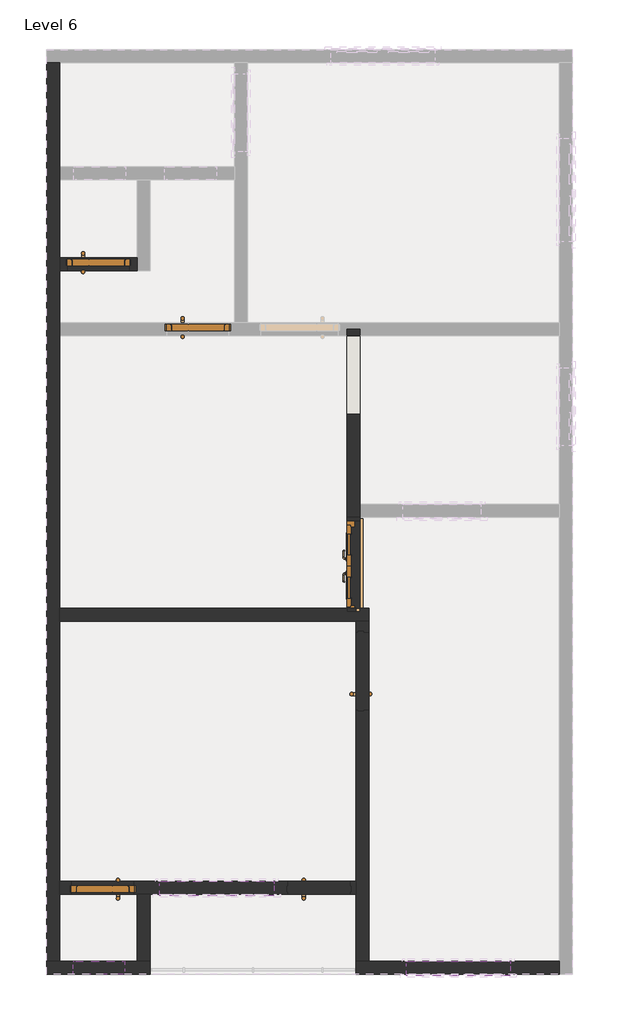
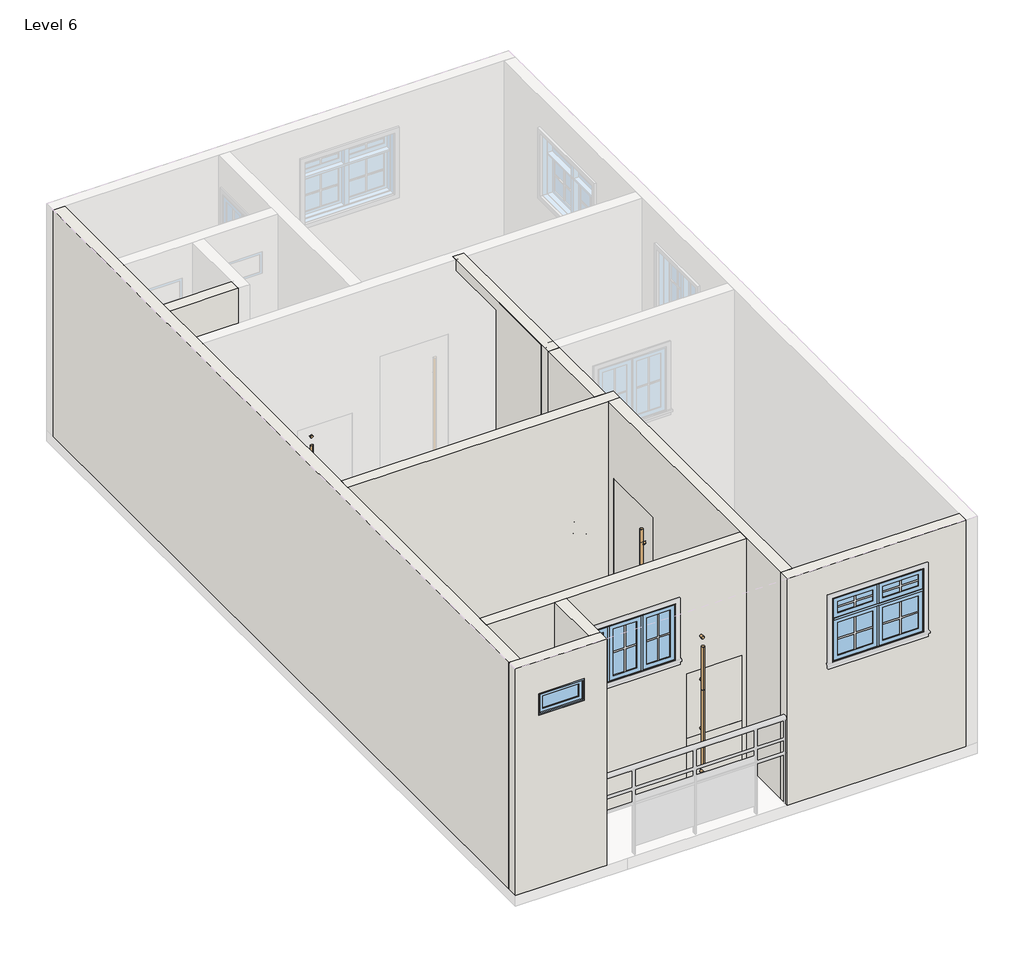
# One storey, part 1 of 3: 31 walls, 7 doors, 6 windows.
"""IFC4 building model written with IfcOpenShell, lengths in millimetres."""

from ifc_helpers import new_model, si_unit, frame, origin, place, context, project, spatial, polyline, outline, extrude, faceted_brep, transform, mapped, element, save
from components import door_9b787682, door_dc81b0c5, door_3_5c4206ef, door_2576ec39, door_55c03dfd, fixed_2_65c13adb, window_61697a4f, m_window_casement_double_awning_double_4_7efa9bbd

model = new_model("IFC4")

# Units and contexts
model_context = context("Model", 3, world=origin())
ifc_project = project(units=[si_unit("LENGTHUNIT", "METRE", prefix="MILLI")], contexts=[model_context])

# Site, building, storey
site = spatial("IfcSite", under=ifc_project)
building = spatial("IfcBuilding", under=site)
storey = spatial("IfcBuildingStorey", under=building, Name="Level 6", Elevation=7010.4)

# Doors
placement = place(None, origin())
door_shape = door_9b787682(model_context)
element("IfcDoor", 1, ObjectType="2'5\"", at=placement, inside=storey, context=model_context, shape_type="MappedRepresentation", body=[
    mapped(door_shape, transform((-22033.2963079, 3049.4742053, 7010.4), x_axis=(1.0, 0.0, 0.0), y_axis=(0.0, 1.0, 0.0), z_axis=(0.0, 0.0, 1.0))),
])
element("IfcDoor", 2, ObjectType="2'5\"", at=placement, inside=storey, context=model_context, shape_type="MappedRepresentation", body=[
    mapped(door_shape, transform((-23201.6963079, 3811.4742053, 7010.4), x_axis=(1.0, 0.0, 0.0), y_axis=(0.0, 1.0, 0.0), z_axis=(0.0, 0.0, 1.0))),
])
element("IfcDoor", 3, ObjectType="2'5\"", at=placement, inside=storey, context=model_context, shape_type="MappedRepresentation", body=[
    mapped(door_shape, transform((-23150.8963079, -3503.7257947, 7010.4), x_axis=(-1.0, 0.0, 0.0), y_axis=(0.0, -1.0, 0.0), z_axis=(0.0, 0.0, 1.0))),
])
door_2_shape = door_dc81b0c5(model_context)
element("IfcDoor", 4, ObjectType="2'5\"", at=placement, inside=storey, context=model_context, shape_type="MappedRepresentation", body=[
    mapped(door_2_shape, transform((-20610.8963079, -3503.7257947, 7056.6445349), x_axis=(1.0, 0.0, 0.0), y_axis=(0.0, 1.0, 0.0), z_axis=(0.0, 0.0, 1.0))),
])
element("IfcDoor", 5, ObjectType="2'5\"", at=placement, inside=storey, context=model_context, shape_type="MappedRepresentation", body=[
    mapped(door_2_shape, transform((-20610.8963079, -3503.7257947, 7666.2445349), x_axis=(1.0, 0.0, 0.0), y_axis=(0.0, 1.0, 0.0), z_axis=(0.0, 0.0, 1.0))),
])
door_3_shape = door_3_5c4206ef(model_context)
element("IfcDoor", 6, ObjectType="3'", at=placement, inside=storey, context=model_context, shape_type="MappedRepresentation", body=[
    mapped(door_3_shape, transform((-20102.8963079, -963.7257947, 7010.4), x_axis=(0.0, 1.0, 0.0), y_axis=(-1.0, 0.0, 0.0), z_axis=(0.0, 0.0, 1.0))),
])
door_4_shape = door_2576ec39(model_context)
door_5_shape = door_55c03dfd(model_context)
element("IfcDoor", 7, ObjectType="ExtDbl (8) : 3'6\"", at=placement, inside=storey, context=model_context, shape_type="MappedRepresentation", body=[
    mapped(door_4_shape, transform((-20204.4963079, 268.1742053, 7010.4), x_axis=(0.0, -1.0, 0.0), y_axis=(1.0, 0.0, 0.0), z_axis=(0.0, 0.0, 1.0))),
    mapped(door_5_shape, transform((-20204.4963079, 268.1742053, 7010.4), x_axis=(0.0, -1.0, 0.0), y_axis=(1.0, 0.0, 0.0), z_axis=(0.0, 0.0, 1.0))),
])

# Walls
element("IfcWall", 8, ObjectType="Generic - 6\"", at=placement, inside=storey, context=model_context, shape_type="Brep", body=[
    faceted_brep([(-17791.4963079, -4367.3257947, 7010.4), (-20026.6963079, -4367.3257947, 7010.4), (-20179.0963079, -4367.3257947, 7010.4), (-20179.0963079, -4367.3257947, 10210.8), (-20026.6963079, -4367.3257947, 10210.8), (-17791.4963079, -4367.3257947, 10210.8), (-19585.5697454, -4367.3257947, 9739.2), (-19585.5697454, -4367.3257947, 8839.2), (-18366.3697454, -4367.3257947, 8839.2), (-18366.3697454, -4367.3257947, 9739.2), (-17791.4963079, -4519.7257947, 7010.4), (-17791.4963079, -4519.7257947, 10210.8), (-20179.0963079, -4519.7257947, 10210.8), (-20179.0963079, -4519.7257947, 7010.4), (-19585.5697454, -4519.7257947, 9739.2), (-18366.3697454, -4519.7257947, 9739.2), (-18366.3697454, -4519.7257947, 8839.2), (-19585.5697454, -4519.7257947, 8839.2)], [[[0, 1, 2, 3, 4, 5], [6, 7, 8, 9]], [[10, 11, 12, 13], [14, 15, 16, 17]], [[2, 1, 0, 10, 13]], [[5, 4, 3, 12, 11]], [[0, 5, 11, 10]], [[3, 2, 13, 12]], [[7, 6, 14, 17]], [[8, 7, 17, 16]], [[9, 8, 16, 15]], [[6, 9, 15, 14]]]),
])
element("IfcWall", 9, ObjectType="Generic - 6\"", at=placement, inside=storey, context=model_context, shape_type="Brep", body=[
    faceted_brep([(-23811.2963079, -4519.7257947, 7010.4), (-22592.0963079, -4519.7257947, 7010.4), (-22592.0963079, -4519.7257947, 10210.8), (-23811.2963079, -4519.7257947, 10210.8), (-23500.5431829, -4519.7257947, 9753.6), (-22890.9431829, -4519.7257947, 9753.6), (-22890.9431829, -4519.7257947, 9448.8), (-23500.5431829, -4519.7257947, 9448.8), (-23811.2963079, -4367.3257947, 7010.4), (-23811.2963079, -4367.3257947, 10210.8), (-23658.8963079, -4367.3257947, 10210.8), (-22744.4963079, -4367.3257947, 10210.8), (-22592.0963079, -4367.3257947, 10210.8), (-22592.0963079, -4367.3257947, 7010.4), (-22744.4963079, -4367.3257947, 7010.4), (-23658.8963079, -4367.3257947, 7010.4), (-23500.5431829, -4367.3257947, 9753.6), (-23500.5431829, -4367.3257947, 9448.8), (-22890.9431829, -4367.3257947, 9448.8), (-22890.9431829, -4367.3257947, 9753.6)], [[[0, 1, 2, 3], [4, 5, 6, 7]], [[8, 9, 10, 11, 12, 13, 14, 15], [16, 17, 18, 19]], [[1, 0, 8, 15, 14, 13]], [[3, 2, 12, 11, 10, 9]], [[0, 3, 9, 8]], [[2, 1, 13, 12]], [[17, 16, 4, 7]], [[18, 17, 7, 6]], [[19, 18, 6, 5]], [[16, 19, 5, 4]]]),
])
element("IfcWall", 10, ObjectType="Generic - 6\"", at=placement, inside=storey, context=model_context, shape_type="Brep", body=[
    faceted_brep([(-23658.8963079, -4367.3257947, 7010.4), (-23658.8963079, -3579.9257947, 7010.4), (-23658.8963079, -3427.5257947, 7010.4), (-23658.8963079, -379.5257947, 7010.4), (-23658.8963079, -227.1257947, 7010.4), (-23658.8963079, 2973.2742053, 7010.4), (-23658.8963079, 3125.6742053, 7010.4), (-23658.8963079, 3735.2742053, 7010.4), (-23658.8963079, 3887.6742053, 7010.4), (-23658.8963079, 4802.0742053, 7010.4), (-23658.8963079, 4954.4742053, 7010.4), (-23658.8963079, 6173.6742053, 7010.4), (-23658.8963079, 6173.6742053, 10210.8), (-23658.8963079, 4954.4742053, 10210.8), (-23658.8963079, 4802.0742053, 10210.8), (-23658.8963079, 3887.6742053, 10210.8), (-23658.8963079, 3735.2742053, 10210.8), (-23658.8963079, 3125.6742053, 10210.8), (-23658.8963079, 2973.2742053, 10210.8), (-23658.8963079, -227.1257947, 10210.8), (-23658.8963079, -379.5257947, 10210.8), (-23658.8963079, -3427.5257947, 10210.8), (-23658.8963079, -3579.9257947, 10210.8), (-23658.8963079, -4367.3257947, 10210.8), (-23811.2963079, -4367.3257947, 7010.4), (-23811.2963079, -4367.3257947, 10210.8), (-23811.2963079, 6173.6742053, 10210.8), (-23811.2963079, 6173.6742053, 7010.4)], [[[0, 1, 2, 3, 4, 5, 6, 7, 8, 9, 10, 11, 12, 13, 14, 15, 16, 17, 18, 19, 20, 21, 22, 23]], [[24, 25, 26, 27]], [[11, 10, 9, 8, 7, 6, 5, 4, 3, 2, 1, 0, 24, 27]], [[23, 22, 21, 20, 19, 18, 17, 16, 15, 14, 13, 12, 26, 25]], [[12, 11, 27, 26]], [[0, 23, 25, 24]]]),
])
element("IfcWall", 11, ObjectType="Generic - 6\"", at=placement, inside=storey, context=model_context, shape_type="Brep", body=[
    faceted_brep([(-20280.6963079, 3049.4742053, 7010.4), (-20280.6963079, 839.6742053, 7010.4), (-20280.6963079, 839.6742053, 10210.8), (-20280.6963079, 3049.4742053, 10210.8), (-20280.6963079, 2974.7724011, 10058.4), (-20280.6963079, 2050.5574639, 10058.4), (-20280.6963079, 2050.5574639, 7620.0), (-20280.6963079, 2974.7724011, 7620.0), (-20128.2963079, 839.6742053, 7010.4), (-20128.2963079, 992.0742053, 7010.4), (-20128.2963079, 3049.4742053, 7010.4), (-20128.2963079, 3049.4742053, 10210.8), (-20128.2963079, 992.0742053, 10210.8), (-20128.2963079, 839.6742053, 10210.8), (-20128.2963079, 2050.5574639, 10058.4), (-20128.2963079, 2974.7724011, 10058.4), (-20128.2963079, 2974.7724011, 7620.0), (-20128.2963079, 2050.5574639, 7620.0)], [[[0, 1, 2, 3], [4, 5, 6, 7]], [[8, 9, 10, 11, 12, 13], [14, 15, 16, 17]], [[1, 0, 10, 9, 8]], [[3, 2, 13, 12, 11]], [[0, 3, 11, 10]], [[2, 1, 8, 13]], [[4, 15, 14, 5]], [[6, 17, 16, 7]], [[15, 4, 7, 16]], [[5, 14, 17, 6]]]),
])
element("IfcWall", 12, ObjectType="Generic - 6\"", at=placement, inside=storey, context=model_context, shape_type="Brep", body=[
    faceted_brep([(-23658.8963079, -379.5257947, 7010.4), (-20179.0963079, -379.5257947, 7010.4), (-20026.6963079, -379.5257947, 7010.4), (-20026.6963079, -379.5257947, 10210.8), (-20179.0963079, -379.5257947, 10210.8), (-23658.8963079, -379.5257947, 10210.8), (-23658.8963079, -227.1257947, 10210.8), (-20280.6963079, -227.1257947, 10210.8), (-20128.2963079, -227.1257947, 10210.8), (-20026.6963079, -227.1257947, 10210.8), (-20026.6963079, -227.1257947, 7010.4), (-20128.2963079, -227.1257947, 7010.4), (-20128.2963079, -227.1257947, 9120.4), (-20280.6963079, -227.1257947, 9120.4), (-20280.6963079, -227.1257947, 7010.4), (-23658.8963079, -227.1257947, 7010.4), (-20280.6963079, -265.2257947, 7010.4), (-20128.2963079, -265.2257947, 7010.4), (-20280.6963079, -265.2257947, 9120.4), (-20128.2963079, -265.2257947, 9120.4)], [[[0, 1, 2, 3, 4, 5]], [[6, 7, 8, 9, 10, 11, 12, 13, 14, 15]], [[2, 1, 0, 15, 14, 16, 17, 11, 10]], [[5, 4, 3, 9, 8, 7, 6]], [[0, 5, 6, 15]], [[3, 2, 10, 9]], [[18, 16, 14, 13]], [[17, 19, 12, 11]], [[19, 18, 13, 12]], [[16, 18, 19, 17]]]),
])
element("IfcWall", 13, ObjectType="Generic - 6\"", at=placement, inside=storey, context=model_context, shape_type="Brep", body=[
    faceted_brep([(-20179.0963079, -4367.3257947, 10210.8), (-20179.0963079, -3579.9257947, 10210.8), (-20179.0963079, -3427.5257947, 10210.8), (-20179.0963079, -379.5257947, 10210.8), (-20179.0963079, -379.5257947, 7010.4), (-20179.0963079, -506.5257947, 7010.4), (-20179.0963079, -506.5257947, 9199.9), (-20179.0963079, -1420.9257947, 9199.9), (-20179.0963079, -1420.9257947, 7010.4), (-20179.0963079, -3427.5257947, 7010.4), (-20179.0963079, -3579.9257947, 7010.4), (-20179.0963079, -4367.3257947, 7010.4), (-20026.6963079, -379.5257947, 10210.8), (-20026.6963079, -4367.3257947, 10210.8), (-20026.6963079, -4367.3257947, 7010.4), (-20026.6963079, -1420.9257947, 7010.4), (-20026.6963079, -1420.9257947, 9199.9), (-20026.6963079, -506.5257947, 9199.9), (-20026.6963079, -506.5257947, 7010.4), (-20026.6963079, -379.5257947, 7010.4), (-20082.0963079, -506.5257947, 7010.4), (-20082.0963079, -491.5257947, 7010.4), (-20159.0963079, -491.5257947, 7010.4), (-20159.0963079, -506.5257947, 7010.4), (-20159.0963079, -1420.9257947, 7010.4), (-20159.0963079, -1435.9257947, 7010.4), (-20082.0963079, -1435.9257947, 7010.4), (-20082.0963079, -1420.9257947, 7010.4), (-20159.0963079, -506.5257947, 9199.9), (-20159.0963079, -1420.9257947, 9199.9), (-20082.0963079, -1420.9257947, 9199.9), (-20082.0963079, -506.5257947, 9199.9), (-20159.0963079, -1435.9257947, 9214.9), (-20159.0963079, -491.5257947, 9214.9), (-20082.0963079, -491.5257947, 9214.9), (-20082.0963079, -1435.9257947, 9214.9)], [[[0, 1, 2, 3, 4, 5, 6, 7, 8, 9, 10, 11]], [[12, 13, 14, 15, 16, 17, 18, 19]], [[4, 19, 18, 20, 21, 22, 23, 5]], [[14, 11, 10, 9, 8, 24, 25, 26, 27, 15]], [[3, 2, 1, 0, 13, 12]], [[0, 11, 14, 13]], [[4, 3, 12, 19]], [[6, 28, 29, 7]], [[16, 30, 31, 17]], [[28, 6, 5, 23]], [[17, 31, 20, 18]], [[7, 29, 24, 8]], [[30, 16, 15, 27]], [[32, 33, 34, 35]], [[34, 33, 22, 21]], [[31, 30, 27, 26, 35, 34, 21, 20]], [[32, 35, 26, 25]], [[29, 28, 23, 22, 33, 32, 25, 24]]]),
])
element("IfcWall", 14, ObjectType="Generic - 6\"", at=placement, inside=storey, context=model_context, shape_type="Brep", body=[
    faceted_brep([(-20179.0963079, -3579.9257947, 10210.8), (-22592.0963079, -3579.9257947, 10210.8), (-22744.4963079, -3579.9257947, 10210.8), (-23658.8963079, -3579.9257947, 10210.8), (-23658.8963079, -3579.9257947, 7010.4), (-23519.1963079, -3579.9257947, 7010.4), (-23519.1963079, -3579.9257947, 8534.4), (-22782.5963079, -3579.9257947, 8534.4), (-22782.5963079, -3579.9257947, 7010.4), (-22744.4963079, -3579.9257947, 7010.4), (-22592.0963079, -3579.9257947, 7010.4), (-20179.0963079, -3579.9257947, 7010.4), (-22484.1463079, -3579.9257947, 8839.2), (-22484.1463079, -3579.9257947, 9639.2), (-21137.9463079, -3579.9257947, 9639.2), (-21137.9463079, -3579.9257947, 8839.2), (-20979.1963079, -3579.9257947, 8580.6445349), (-20242.5963079, -3579.9257947, 8580.6445349), (-20242.5963079, -3579.9257947, 7056.6445349), (-20979.1963079, -3579.9257947, 7056.6445349), (-23658.8963079, -3427.5257947, 10210.8), (-20179.0963079, -3427.5257947, 10210.8), (-20179.0963079, -3427.5257947, 7010.4), (-22782.5963079, -3427.5257947, 7010.4), (-22782.5963079, -3427.5257947, 8534.4), (-23519.1963079, -3427.5257947, 8534.4), (-23519.1963079, -3427.5257947, 7010.4), (-23658.8963079, -3427.5257947, 7010.4), (-22484.1463079, -3427.5257947, 9639.2), (-22484.1463079, -3427.5257947, 8839.2), (-21137.9463079, -3427.5257947, 8839.2), (-21137.9463079, -3427.5257947, 9639.2), (-20242.5963079, -3427.5257947, 8580.6445349), (-20979.1963079, -3427.5257947, 8580.6445349), (-20979.1963079, -3427.5257947, 7056.6445349), (-20242.5963079, -3427.5257947, 7056.6445349), (-23519.1963079, -3482.9257947, 7010.4), (-23534.1963079, -3482.9257947, 7010.4), (-23534.1963079, -3559.9257947, 7010.4), (-23519.1963079, -3559.9257947, 7010.4), (-22782.5963079, -3559.9257947, 7010.4), (-22767.5963079, -3559.9257947, 7010.4), (-22767.5963079, -3482.9257947, 7010.4), (-22782.5963079, -3482.9257947, 7010.4), (-20979.1963079, -3559.9257947, 8580.6445349), (-20242.5963079, -3559.9257947, 8580.6445349), (-20242.5963079, -3482.9257947, 8580.6445349), (-20979.1963079, -3482.9257947, 8580.6445349), (-20242.5963079, -3559.9257947, 7056.6445349), (-20242.5963079, -3482.9257947, 7056.6445349), (-20227.5963079, -3559.9257947, 7056.6445349), (-20227.5963079, -3482.9257947, 7056.6445349), (-20979.1963079, -3482.9257947, 7056.6445349), (-20994.1963079, -3482.9257947, 7056.6445349), (-20994.1963079, -3559.9257947, 7056.6445349), (-20979.1963079, -3559.9257947, 7056.6445349), (-20994.1963079, -3559.9257947, 8595.6445349), (-20994.1963079, -3482.9257947, 8595.6445349), (-20227.5963079, -3482.9257947, 8595.6445349), (-20227.5963079, -3559.9257947, 8595.6445349), (-23519.1963079, -3559.9257947, 8534.4), (-22782.5963079, -3559.9257947, 8534.4), (-22782.5963079, -3482.9257947, 8534.4), (-23519.1963079, -3482.9257947, 8534.4), (-22767.5963079, -3559.9257947, 8549.4), (-23534.1963079, -3559.9257947, 8549.4), (-23534.1963079, -3482.9257947, 8549.4), (-22767.5963079, -3482.9257947, 8549.4)], [[[0, 1, 2, 3, 4, 5, 6, 7, 8, 9, 10, 11], [12, 13, 14, 15], [16, 17, 18, 19]], [[20, 21, 22, 23, 24, 25, 26, 27], [28, 29, 30, 31], [32, 33, 34, 35]], [[4, 27, 26, 36, 37, 38, 39, 5]], [[22, 11, 10, 9, 8, 40, 41, 42, 43, 23]], [[3, 2, 1, 0, 21, 20]], [[4, 3, 20, 27]], [[0, 11, 22, 21]], [[29, 28, 13, 12]], [[30, 29, 12, 15]], [[31, 30, 15, 14]], [[28, 31, 14, 13]], [[16, 44, 45, 17]], [[32, 46, 47, 33]], [[17, 45, 48, 18]], [[46, 32, 35, 49]], [[18, 48, 50, 51, 49, 35, 34, 52, 53, 54, 55, 19]], [[44, 16, 19, 55]], [[33, 47, 52, 34]], [[56, 57, 58, 59]], [[51, 50, 59, 58]], [[47, 46, 49, 51, 58, 57, 53, 52]], [[54, 53, 57, 56]], [[45, 44, 55, 54, 56, 59, 50, 48]], [[6, 60, 61, 7]], [[24, 62, 63, 25]], [[60, 6, 5, 39]], [[25, 63, 36, 26]], [[7, 61, 40, 8]], [[62, 24, 23, 43]], [[64, 65, 66, 67]], [[66, 65, 38, 37]], [[63, 62, 43, 42, 67, 66, 37, 36]], [[64, 67, 42, 41]], [[61, 60, 39, 38, 65, 64, 41, 40]]]),
])
element("IfcWall", 15, ObjectType="Generic - 6\"", at=placement, inside=storey, context=model_context, shape_type="SweptSolid", body=[
    extrude(outline(polyline([(-22744.4963079, -4367.3257947), (-22744.4963079, -3579.9257947), (-22592.0963079, -3579.9257947), (-22592.0963079, -4367.3257947), (-22744.4963079, -4367.3257947)])), frame((0.0, 0.0, 7010.4), z_axis=(0.0, 0.0, 1.0), x_axis=(1.0, 0.0, 0.0)), (0.0, 0.0, 1.0), 3200.4),
])
element("IfcWall", 16, ObjectType="Generic - 6\"", at=placement, inside=storey, context=model_context, shape_type="Brep", body=[
    faceted_brep([(-22744.4963079, 3735.2742053, 10210.8), (-23658.8963079, 3735.2742053, 10210.8), (-23658.8963079, 3735.2742053, 7010.4), (-23569.9963079, 3735.2742053, 7010.4), (-23569.9963079, 3735.2742053, 8534.4), (-22833.3963079, 3735.2742053, 8534.4), (-22833.3963079, 3735.2742053, 7010.4), (-22744.4963079, 3735.2742053, 7010.4), (-23658.8963079, 3887.6742053, 10210.8), (-22744.4963079, 3887.6742053, 10210.8), (-22744.4963079, 3887.6742053, 7010.4), (-22833.3963079, 3887.6742053, 7010.4), (-22833.3963079, 3887.6742053, 8534.4), (-23569.9963079, 3887.6742053, 8534.4), (-23569.9963079, 3887.6742053, 7010.4), (-23658.8963079, 3887.6742053, 7010.4), (-23569.9963079, 3867.6742053, 7010.4), (-23584.9963079, 3867.6742053, 7010.4), (-23584.9963079, 3790.6742053, 7010.4), (-23569.9963079, 3790.6742053, 7010.4), (-22833.3963079, 3790.6742053, 7010.4), (-22818.3963079, 3790.6742053, 7010.4), (-22818.3963079, 3867.6742053, 7010.4), (-22833.3963079, 3867.6742053, 7010.4), (-22833.3963079, 3867.6742053, 8534.4), (-23569.9963079, 3867.6742053, 8534.4), (-23569.9963079, 3790.6742053, 8534.4), (-22833.3963079, 3790.6742053, 8534.4), (-23584.9963079, 3867.6742053, 8549.4), (-22818.3963079, 3867.6742053, 8549.4), (-22818.3963079, 3790.6742053, 8549.4), (-23584.9963079, 3790.6742053, 8549.4)], [[[0, 1, 2, 3, 4, 5, 6, 7]], [[8, 9, 10, 11, 12, 13, 14, 15]], [[2, 15, 14, 16, 17, 18, 19, 3]], [[10, 7, 6, 20, 21, 22, 23, 11]], [[1, 0, 9, 8]], [[0, 7, 10, 9]], [[2, 1, 8, 15]], [[12, 24, 25, 13]], [[4, 26, 27, 5]], [[24, 12, 11, 23]], [[5, 27, 20, 6]], [[13, 25, 16, 14]], [[26, 4, 3, 19]], [[28, 29, 30, 31]], [[30, 29, 22, 21]], [[27, 26, 19, 18, 31, 30, 21, 20]], [[28, 31, 18, 17]], [[25, 24, 23, 22, 29, 28, 17, 16]]]),
])
element("IfcWall", 17, ObjectType="Generic - 6\"", at=placement, inside=storey, context=model_context, shape_type="SweptSolid", body=[
    extrude(outline(polyline([(-227.1257947, 10210.8), (839.6742053, 10210.8), (839.6742053, 7010.4), (801.5742053, 7010.4), (801.5742053, 9120.4), (-227.1257947, 9120.4), (-227.1257947, 10210.8)])), frame((-20280.6963079, 0.0, 0.0), z_axis=(1.0, 0.0, 0.0), x_axis=(0.0, 1.0, 0.0)), (0.0, 0.0, 1.0), 152.4),
])
element("IfcWall", 18, ObjectType="Generic - 6\"", at=placement, inside=storey, context=model_context, shape_type="SweptSolid", body=[
    extrude(outline(polyline([(3049.4742053, 7010.4), (992.0742053, 7010.4), (992.0742053, 10210.8), (3049.4742053, 10210.8), (3049.4742053, 7010.4)]), holes=[polyline([(2974.7724011, 10058.4), (2050.5574639, 10058.4), (2050.5574639, 7620.0), (2974.7724011, 7620.0), (2974.7724011, 10058.4)])]), frame((-20280.6963079, 0.0, 0.0), z_axis=(1.0, 0.0, 0.0), x_axis=(0.0, 1.0, 0.0)), (0.0, 0.0, 1.0), 152.4),
])
element("IfcWall", 19, ObjectType="Generic - 6\"", at=placement, inside=storey, context=model_context, shape_type="Brep", body=[
    faceted_brep([(-23658.8963079, -379.5257947, 7010.4), (-20179.0963079, -379.5257947, 7010.4), (-20179.0963079, -379.5257947, 10210.8), (-23658.8963079, -379.5257947, 10210.8), (-23658.8963079, -227.1257947, 7010.4), (-23658.8963079, -227.1257947, 10210.8), (-20280.6963079, -227.1257947, 10210.8), (-20179.0963079, -227.1257947, 10210.8), (-20179.0963079, -227.1257947, 7010.4), (-20280.6963079, -227.1257947, 7010.4)], [[[0, 1, 2, 3]], [[4, 5, 6, 7, 8, 9]], [[1, 0, 4, 9, 8]], [[3, 2, 7, 6, 5]], [[2, 1, 8, 7]], [[0, 3, 5, 4]]]),
])
element("IfcWall", 20, ObjectType="Generic - 6\"", at=placement, inside=storey, context=model_context, shape_type="Brep", body=[
    faceted_brep([(-20179.0963079, -379.5257947, 7010.4), (-20179.0963079, -3427.5257947, 7010.4), (-20179.0963079, -3579.9257947, 7010.4), (-20179.0963079, -4367.3257947, 7010.4), (-20179.0963079, -4367.3257947, 10210.8), (-20179.0963079, -3579.9257947, 10210.8), (-20179.0963079, -3427.5257947, 10210.8), (-20179.0963079, -379.5257947, 10210.8), (-20026.6963079, -379.5257947, 7010.4), (-20026.6963079, -379.5257947, 10210.8), (-20026.6963079, -4367.3257947, 10210.8), (-20026.6963079, -4367.3257947, 7010.4)], [[[0, 1, 2, 3, 4, 5, 6, 7]], [[8, 9, 10, 11]], [[3, 2, 1, 0, 8, 11]], [[7, 6, 5, 4, 10, 9]], [[4, 3, 11, 10]], [[0, 7, 9, 8]]]),
])
element("IfcWall", 21, ObjectType="Generic - 6\"", at=placement, inside=storey, context=model_context, shape_type="Brep", body=[
    faceted_brep([(-23658.8963079, -3579.9257947, 7010.4), (-22744.4963079, -3579.9257947, 7010.4), (-22592.0963079, -3579.9257947, 7010.4), (-20179.0963079, -3579.9257947, 7010.4), (-20179.0963079, -3579.9257947, 10210.8), (-22592.0963079, -3579.9257947, 10210.8), (-22744.4963079, -3579.9257947, 10210.8), (-23658.8963079, -3579.9257947, 10210.8), (-22484.1463079, -3579.9257947, 8839.2), (-22484.1463079, -3579.9257947, 9639.2), (-21137.9463079, -3579.9257947, 9639.2), (-21137.9463079, -3579.9257947, 8839.2), (-20979.1963079, -3579.9257947, 9190.2445349), (-20242.5963079, -3579.9257947, 9190.2445349), (-20242.5963079, -3579.9257947, 7666.2445349), (-20979.1963079, -3579.9257947, 7666.2445349), (-20179.0963079, -3427.5257947, 7010.4), (-23658.8963079, -3427.5257947, 7010.4), (-23658.8963079, -3427.5257947, 10210.8), (-20179.0963079, -3427.5257947, 10210.8), (-22484.1463079, -3427.5257947, 9639.2), (-22484.1463079, -3427.5257947, 8839.2), (-21137.9463079, -3427.5257947, 8839.2), (-21137.9463079, -3427.5257947, 9639.2), (-20242.5963079, -3427.5257947, 9190.2445349), (-20979.1963079, -3427.5257947, 9190.2445349), (-20979.1963079, -3427.5257947, 7666.2445349), (-20242.5963079, -3427.5257947, 7666.2445349), (-20979.1963079, -3559.9257947, 9190.2445349), (-20242.5963079, -3559.9257947, 9190.2445349), (-20242.5963079, -3482.9257947, 9190.2445349), (-20979.1963079, -3482.9257947, 9190.2445349), (-20242.5963079, -3559.9257947, 7666.2445349), (-20242.5963079, -3482.9257947, 7666.2445349), (-20227.5963079, -3559.9257947, 7666.2445349), (-20227.5963079, -3482.9257947, 7666.2445349), (-20979.1963079, -3482.9257947, 7666.2445349), (-20994.1963079, -3482.9257947, 7666.2445349), (-20994.1963079, -3559.9257947, 7666.2445349), (-20979.1963079, -3559.9257947, 7666.2445349), (-20994.1963079, -3559.9257947, 9205.2445349), (-20994.1963079, -3482.9257947, 9205.2445349), (-20227.5963079, -3482.9257947, 9205.2445349), (-20227.5963079, -3559.9257947, 9205.2445349)], [[[0, 1, 2, 3, 4, 5, 6, 7], [8, 9, 10, 11], [12, 13, 14, 15]], [[16, 17, 18, 19], [20, 21, 22, 23], [24, 25, 26, 27]], [[3, 2, 1, 0, 17, 16]], [[7, 6, 5, 4, 19, 18]], [[4, 3, 16, 19]], [[21, 20, 9, 8]], [[22, 21, 8, 11]], [[23, 22, 11, 10]], [[20, 23, 10, 9]], [[12, 28, 29, 13]], [[24, 30, 31, 25]], [[13, 29, 32, 14]], [[30, 24, 27, 33]], [[14, 32, 34, 35, 33, 27, 26, 36, 37, 38, 39, 15]], [[28, 12, 15, 39]], [[25, 31, 36, 26]], [[40, 41, 42, 43]], [[35, 34, 43, 42]], [[31, 30, 33, 35, 42, 41, 37, 36]], [[38, 37, 41, 40]], [[29, 28, 39, 38, 40, 43, 34, 32]], [[0, 7, 18, 17]]]),
])
element("IfcWall", 22, ObjectType="Generic - 6\"", at=placement, inside=storey, context=model_context, shape_type="SweptSolid", body=[
    extrude(outline(polyline([(-22744.4963079, -4367.3257947), (-22744.4963079, -3579.9257947), (-22592.0963079, -3579.9257947), (-22592.0963079, -4367.3257947), (-22744.4963079, -4367.3257947)])), frame((0.0, 0.0, 7010.4), z_axis=(0.0, 0.0, 1.0), x_axis=(1.0, 0.0, 0.0)), (0.0, 0.0, 1.0), 3200.4),
])
element("IfcWall", 23, ObjectType="Generic - 6\"", at=placement, inside=storey, context=model_context, shape_type="SweptSolid", body=[
    extrude(outline(polyline([(-22744.4963079, 3735.2742053), (-23658.8963079, 3735.2742053), (-23658.8963079, 3887.6742053), (-22744.4963079, 3887.6742053), (-22744.4963079, 3735.2742053)])), frame((0.0, 0.0, 7010.4), z_axis=(0.0, 0.0, 1.0), x_axis=(1.0, 0.0, 0.0)), (0.0, 0.0, 1.0), 3200.4),
])
element("IfcWall", 24, ObjectType="Generic - 6\"", at=placement, inside=storey, context=model_context, shape_type="Brep", body=[
    faceted_brep([(-20280.6963079, 839.6742053, 7010.4), (-20280.6963079, -227.1257947, 7010.4), (-20280.6963079, -227.1257947, 10210.8), (-20280.6963079, 839.6742053, 10210.8), (-20128.2963079, 839.6742053, 7010.4), (-20128.2963079, 839.6742053, 10210.8), (-20128.2963079, -227.1257947, 10210.8), (-20128.2963079, -227.1257947, 7010.4), (-20179.0963079, -227.1257947, 10210.8)], [[[0, 1, 2, 3]], [[4, 5, 6, 7]], [[1, 0, 4, 7]], [[3, 2, 8, 6, 5]], [[2, 1, 7, 6, 8]], [[0, 3, 5, 4]]]),
])
element("IfcWall", 25, ObjectType="Generic - 6\"", at=placement, inside=storey, context=model_context, shape_type="SweptSolid", body=[
    extrude(outline(polyline([(3049.4742053, 7010.4), (915.8742053, 7010.4), (915.8742053, 10210.8), (3049.4742053, 10210.8), (3049.4742053, 7010.4)]), holes=[polyline([(2974.7724011, 10058.4), (2050.5574639, 10058.4), (2050.5574639, 7620.0), (2974.7724011, 7620.0), (2974.7724011, 10058.4)])]), frame((-20280.6963079, 0.0, 0.0), z_axis=(1.0, 0.0, 0.0), x_axis=(0.0, 1.0, 0.0)), (0.0, 0.0, 1.0), 152.4),
])
element("IfcWall", 26, ObjectType="Generic - 6\"", at=placement, inside=storey, context=model_context, shape_type="Brep", body=[
    faceted_brep([(-23658.8963079, -379.5257947, 7010.4), (-20179.0963079, -379.5257947, 7010.4), (-20179.0963079, -379.5257947, 10210.8), (-23658.8963079, -379.5257947, 10210.8), (-23658.8963079, -227.1257947, 7010.4), (-23658.8963079, -227.1257947, 10210.8), (-20280.6963079, -227.1257947, 10210.8), (-20179.0963079, -227.1257947, 10210.8), (-20179.0963079, -227.1257947, 7010.4), (-20280.6963079, -227.1257947, 7010.4)], [[[0, 1, 2, 3]], [[4, 5, 6, 7, 8, 9]], [[1, 0, 4, 9, 8]], [[3, 2, 7, 6, 5]], [[2, 1, 8, 7]], [[0, 3, 5, 4]]]),
])
element("IfcWall", 27, ObjectType="Generic - 6\"", at=placement, inside=storey, context=model_context, shape_type="Brep", body=[
    faceted_brep([(-20179.0963079, -379.5257947, 7010.4), (-20179.0963079, -3427.5257947, 7010.4), (-20179.0963079, -3579.9257947, 7010.4), (-20179.0963079, -4367.3257947, 7010.4), (-20179.0963079, -4367.3257947, 10210.8), (-20179.0963079, -3579.9257947, 10210.8), (-20179.0963079, -3427.5257947, 10210.8), (-20179.0963079, -379.5257947, 10210.8), (-20026.6963079, -379.5257947, 7010.4), (-20026.6963079, -379.5257947, 10210.8), (-20026.6963079, -4367.3257947, 10210.8), (-20026.6963079, -4367.3257947, 7010.4)], [[[0, 1, 2, 3, 4, 5, 6, 7]], [[8, 9, 10, 11]], [[3, 2, 1, 0, 8, 11]], [[7, 6, 5, 4, 10, 9]], [[4, 3, 11, 10]], [[0, 7, 9, 8]]]),
])
element("IfcWall", 28, ObjectType="Generic - 6\"", at=placement, inside=storey, context=model_context, shape_type="Brep", body=[
    faceted_brep([(-23658.8963079, -3579.9257947, 7010.4), (-22744.4963079, -3579.9257947, 7010.4), (-22592.0963079, -3579.9257947, 7010.4), (-20179.0963079, -3579.9257947, 7010.4), (-20179.0963079, -3579.9257947, 10210.8), (-22592.0963079, -3579.9257947, 10210.8), (-22744.4963079, -3579.9257947, 10210.8), (-23658.8963079, -3579.9257947, 10210.8), (-22484.1463079, -3579.9257947, 9639.2), (-21137.9463079, -3579.9257947, 9639.2), (-21137.9463079, -3579.9257947, 8839.2), (-22484.1463079, -3579.9257947, 8839.2), (-23658.8963079, -3427.5257947, 7010.4), (-23658.8963079, -3427.5257947, 10210.8), (-20179.0963079, -3427.5257947, 10210.8), (-20179.0963079, -3427.5257947, 7010.4), (-22484.1463079, -3427.5257947, 9639.2), (-22484.1463079, -3427.5257947, 8839.2), (-21137.9463079, -3427.5257947, 8839.2), (-21137.9463079, -3427.5257947, 9639.2)], [[[0, 1, 2, 3, 4, 5, 6, 7], [8, 9, 10, 11]], [[12, 13, 14, 15], [16, 17, 18, 19]], [[3, 2, 1, 0, 12, 15]], [[7, 6, 5, 4, 14, 13]], [[4, 3, 15, 14]], [[17, 16, 8, 11]], [[18, 17, 11, 10]], [[19, 18, 10, 9]], [[16, 19, 9, 8]], [[0, 7, 13, 12]]]),
])
element("IfcWall", 29, ObjectType="Generic - 6\"", at=placement, inside=storey, context=model_context, shape_type="SweptSolid", body=[
    extrude(outline(polyline([(-22744.4963079, -4367.3257947), (-22744.4963079, -3579.9257947), (-22592.0963079, -3579.9257947), (-22592.0963079, -4367.3257947), (-22744.4963079, -4367.3257947)])), frame((0.0, 0.0, 7010.4), z_axis=(0.0, 0.0, 1.0), x_axis=(1.0, 0.0, 0.0)), (0.0, 0.0, 1.0), 3200.4),
])
element("IfcWall", 30, ObjectType="Generic - 6\"", at=placement, inside=storey, context=model_context, shape_type="SweptSolid", body=[
    extrude(outline(polyline([(-22744.4963079, 3735.2742053), (-23658.8963079, 3735.2742053), (-23658.8963079, 3887.6742053), (-22744.4963079, 3887.6742053), (-22744.4963079, 3735.2742053)])), frame((0.0, 0.0, 7010.4), z_axis=(0.0, 0.0, 1.0), x_axis=(1.0, 0.0, 0.0)), (0.0, 0.0, 1.0), 3200.4),
])
element("IfcWall", 31, ObjectType="Generic - 6\"", at=placement, inside=storey, context=model_context, shape_type="Brep", body=[
    faceted_brep([(-20280.6963079, 839.6742053, 7010.4), (-20280.6963079, -227.1257947, 7010.4), (-20280.6963079, -227.1257947, 10210.8), (-20280.6963079, 839.6742053, 10210.8), (-20128.2963079, 839.6742053, 7010.4), (-20128.2963079, 839.6742053, 10210.8), (-20128.2963079, -227.1257947, 10210.8), (-20128.2963079, -227.1257947, 7010.4), (-20179.0963079, -227.1257947, 10210.8)], [[[0, 1, 2, 3]], [[4, 5, 6, 7]], [[1, 0, 4, 7]], [[3, 2, 8, 6, 5]], [[2, 1, 7, 6, 8]], [[0, 3, 5, 4]]]),
])
element("IfcWall", 32, ObjectType="Generic - 6\"", at=placement, inside=storey, context=model_context, shape_type="SweptSolid", body=[
    extrude(outline(polyline([(3049.4742053, 7010.4), (992.0742053, 7010.4), (992.0742053, 10210.8), (3049.4742053, 10210.8), (3049.4742053, 7010.4)]), holes=[polyline([(2974.7724011, 10058.4), (2050.5574639, 10058.4), (2050.5574639, 7620.0), (2974.7724011, 7620.0), (2974.7724011, 10058.4)])]), frame((-20280.6963079, 0.0, 0.0), z_axis=(1.0, 0.0, 0.0), x_axis=(0.0, 1.0, 0.0)), (0.0, 0.0, 1.0), 152.4),
])
element("IfcWall", 33, ObjectType="Generic - 6\"", at=placement, inside=storey, context=model_context, shape_type="Brep", body=[
    faceted_brep([(-23658.8963079, -379.5257947, 7010.4), (-20179.0963079, -379.5257947, 7010.4), (-20179.0963079, -379.5257947, 10210.8), (-23658.8963079, -379.5257947, 10210.8), (-23658.8963079, -227.1257947, 7010.4), (-23658.8963079, -227.1257947, 10210.8), (-20280.6963079, -227.1257947, 10210.8), (-20179.0963079, -227.1257947, 10210.8), (-20179.0963079, -227.1257947, 7010.4), (-20280.6963079, -227.1257947, 7010.4)], [[[0, 1, 2, 3]], [[4, 5, 6, 7, 8, 9]], [[1, 0, 4, 9, 8]], [[3, 2, 7, 6, 5]], [[2, 1, 8, 7]], [[0, 3, 5, 4]]]),
])
element("IfcWall", 34, ObjectType="Generic - 6\"", at=placement, inside=storey, context=model_context, shape_type="Brep", body=[
    faceted_brep([(-20179.0963079, -379.5257947, 7010.4), (-20179.0963079, -3427.5257947, 7010.4), (-20179.0963079, -3579.9257947, 7010.4), (-20179.0963079, -4367.3257947, 7010.4), (-20179.0963079, -4367.3257947, 10210.8), (-20179.0963079, -3579.9257947, 10210.8), (-20179.0963079, -3427.5257947, 10210.8), (-20179.0963079, -379.5257947, 10210.8), (-20026.6963079, -379.5257947, 7010.4), (-20026.6963079, -379.5257947, 10210.8), (-20026.6963079, -4367.3257947, 10210.8), (-20026.6963079, -4367.3257947, 7010.4)], [[[0, 1, 2, 3, 4, 5, 6, 7]], [[8, 9, 10, 11]], [[3, 2, 1, 0, 8, 11]], [[7, 6, 5, 4, 10, 9]], [[4, 3, 11, 10]], [[0, 7, 9, 8]]]),
])
element("IfcWall", 35, ObjectType="Generic - 6\"", at=placement, inside=storey, context=model_context, shape_type="Brep", body=[
    faceted_brep([(-23658.8963079, -3579.9257947, 7010.4), (-22744.4963079, -3579.9257947, 7010.4), (-22592.0963079, -3579.9257947, 7010.4), (-20179.0963079, -3579.9257947, 7010.4), (-20179.0963079, -3579.9257947, 10210.8), (-22592.0963079, -3579.9257947, 10210.8), (-22744.4963079, -3579.9257947, 10210.8), (-23658.8963079, -3579.9257947, 10210.8), (-22484.1463079, -3579.9257947, 8839.2), (-22484.1463079, -3579.9257947, 9639.2), (-21137.9463079, -3579.9257947, 9639.2), (-21137.9463079, -3579.9257947, 8839.2), (-20179.0963079, -3427.5257947, 7010.4), (-23658.8963079, -3427.5257947, 7010.4), (-23658.8963079, -3427.5257947, 10210.8), (-20179.0963079, -3427.5257947, 10210.8), (-22484.1463079, -3427.5257947, 9639.2), (-22484.1463079, -3427.5257947, 8839.2), (-21137.9463079, -3427.5257947, 8839.2), (-21137.9463079, -3427.5257947, 9639.2)], [[[0, 1, 2, 3, 4, 5, 6, 7], [8, 9, 10, 11]], [[12, 13, 14, 15], [16, 17, 18, 19]], [[3, 2, 1, 0, 13, 12]], [[7, 6, 5, 4, 15, 14]], [[4, 3, 12, 15]], [[17, 16, 9, 8]], [[18, 17, 8, 11]], [[19, 18, 11, 10]], [[16, 19, 10, 9]], [[0, 7, 14, 13]]]),
])
element("IfcWall", 36, ObjectType="Generic - 6\"", at=placement, inside=storey, context=model_context, shape_type="SweptSolid", body=[
    extrude(outline(polyline([(-22744.4963079, -4367.3257947), (-22744.4963079, -3579.9257947), (-22592.0963079, -3579.9257947), (-22592.0963079, -4367.3257947), (-22744.4963079, -4367.3257947)])), frame((0.0, 0.0, 7010.4), z_axis=(0.0, 0.0, 1.0), x_axis=(1.0, 0.0, 0.0)), (0.0, 0.0, 1.0), 3200.4),
])
element("IfcWall", 37, ObjectType="Generic - 6\"", at=placement, inside=storey, context=model_context, shape_type="SweptSolid", body=[
    extrude(outline(polyline([(-22744.4963079, 3735.2742053), (-23658.8963079, 3735.2742053), (-23658.8963079, 3887.6742053), (-22744.4963079, 3887.6742053), (-22744.4963079, 3735.2742053)])), frame((0.0, 0.0, 7010.4), z_axis=(0.0, 0.0, 1.0), x_axis=(1.0, 0.0, 0.0)), (0.0, 0.0, 1.0), 3200.4),
])
element("IfcWall", 38, ObjectType="Generic - 6\"", at=placement, inside=storey, context=model_context, shape_type="Brep", body=[
    faceted_brep([(-20280.6963079, 839.6742053, 7010.4), (-20280.6963079, -227.1257947, 7010.4), (-20280.6963079, -227.1257947, 10210.8), (-20280.6963079, 839.6742053, 10210.8), (-20128.2963079, 839.6742053, 7010.4), (-20128.2963079, 839.6742053, 10210.8), (-20128.2963079, -227.1257947, 10210.8), (-20128.2963079, -227.1257947, 7010.4), (-20179.0963079, -227.1257947, 7010.4), (-20179.0963079, -227.1257947, 10210.8)], [[[0, 1, 2, 3]], [[4, 5, 6, 7]], [[1, 0, 4, 7, 8]], [[3, 2, 9, 6, 5]], [[2, 1, 8, 7, 6, 9]], [[0, 3, 5, 4]]]),
])

# Windows
fixed_2_shape = fixed_2_65c13adb(model_context)
element("IfcWindow", 39, ObjectType="Fixed : 2'", at=placement, inside=storey, context=model_context, shape_type="MappedRepresentation", body=[
    mapped(fixed_2_shape, transform((-23233.8431829, -4443.5257947, 8534.4), x_axis=(-1.0, 0.0, 0.0), y_axis=(0.0, -1.0, 0.0), z_axis=(0.0, 0.0, 1.0))),
])
window_shape = window_61697a4f(model_context)
element("IfcWindow", 40, ObjectType="M_Window-Awning-Triple-Horizontal : 4'5\"", at=placement, inside=storey, context=model_context, shape_type="MappedRepresentation", body=[
    mapped(window_shape, transform((-21811.0463079, -3503.7257947, 7939.2), x_axis=(-1.0, 0.0, 0.0), y_axis=(0.0, -1.0, 0.0), z_axis=(0.0, 0.0, 1.0))),
])
element("IfcWindow", 41, ObjectType="M_Window-Awning-Triple-Horizontal : 4'5\"", at=placement, inside=storey, context=model_context, shape_type="MappedRepresentation", body=[
    mapped(window_shape, transform((-21811.0463079, -3503.7257947, 7939.2), x_axis=(-1.0, 0.0, 0.0), y_axis=(0.0, -1.0, 0.0), z_axis=(0.0, 0.0, 1.0))),
])
element("IfcWindow", 42, ObjectType="M_Window-Awning-Triple-Horizontal : 4'5\"", at=placement, inside=storey, context=model_context, shape_type="MappedRepresentation", body=[
    mapped(window_shape, transform((-21811.0463079, -3503.7257947, 7939.2), x_axis=(-1.0, 0.0, 0.0), y_axis=(0.0, -1.0, 0.0), z_axis=(0.0, 0.0, 1.0))),
])
element("IfcWindow", 43, ObjectType="M_Window-Awning-Triple-Horizontal : 4'5\"", at=placement, inside=storey, context=model_context, shape_type="MappedRepresentation", body=[
    mapped(window_shape, transform((-21811.0463079, -3503.7257947, 7939.2), x_axis=(-1.0, 0.0, 0.0), y_axis=(0.0, -1.0, 0.0), z_axis=(0.0, 0.0, 1.0))),
])
m_window_casement_double_awning_double_4_shape = m_window_casement_double_awning_double_4_7efa9bbd(model_context)
element("IfcWindow", 44, ObjectType="M_Window-Casement-Double-Awning-Double : 4'", at=placement, inside=storey, context=model_context, shape_type="MappedRepresentation", body=[
    mapped(m_window_casement_double_awning_double_4_shape, transform((-18975.9697454, -4443.5257947, 7939.2), x_axis=(-1.0, 0.0, 0.0), y_axis=(0.0, -1.0, 0.0), z_axis=(0.0, 0.0, 1.0))),
])

save(model, "model.ifc")

# Revit data of these elements
# Type "2'5\""
#   Type Mark = "9"
#   Water resistance = "up to Class E900, EN 12208:2001"
#   Uniclass2015Version = "v1.21"
#   Uniclass2015Reference = "Ss_25_30_20_30"
#   Uniclass2015Description = "Frame and door leaf system"
#   URL = "www.aluprof.com"
#   Type IFC Predefined Type = "USERDEFINED"
#   Right-hand / Left-hand door [instance default] = ""
#   Resistance to wind load = "up to Class C5/B5, EN 12210:2001"
#   Insert type = "ST"
#   Hardware [instance default] = ""
#   Product page = "https://aluprof.com/en/architects/offer/window-and-door-systems/panel-doors#visualisation"
#   Operation = "SinglePanelOutwardOpening"
#   Opening type = "Outward"
#   NBSReference = "25-50-20/125"
#   NBSDescription = "Frame and door leaf system"
#   Important = "The actual acceptable construction dimensions are dependent on the selection of profiles and hardware, glazing type, construction weight and the construction’s operating conditions. These should be determined by a suitably qualified person, and using ALUPROF’s calculation software"
#   IfcExportType = "USERDEFINED"
#   IfcExportAs = "IfcDoorType"
#   Handle type [instance default] = ""
#   Manufacturer = "ALUPROF SA"
#   Export Type to IFC As = "IfcDoorType"
#   Door sill type [instance default] = ""
#   Description = "External single-leaf panel door outward opening"
#   Model = "MB-86 ST Panel Door AD07"
#   Content of the recyclate in the material = "69.2%"
#   COBie.Type.WarrantyDurationParts = ""
#   COBie.Type.Name = ""
#   COBie.Type.Manufacturer = "ALUPROF SA"
#   COBie.Space.Name = ""
#   COBie.Floor.Name = ""
#   COBie.Facility.Name = ""
#   COBie.CreatedOn = ""
#   COBie.Component.WarrantyStartDate = ""
#   COBie.Component.Name = "MB-86 ST Panel Door AD07"
#   Burglar resistance = "RC2"
#   Air permeability = "up to Class 4, EN 12207:2001"
#   Width of the active leaf = 2' - 1.17717"
#   Placement in wall = 0' - 0.7874"
#   Thickness = 0' - 3.0315"
#   Height of the opening sash = 4' - 9.44094"
#   Handle Offset = 3' - 5.33858"
#   Rough Height = 5' - 2.40945"
#   Rough Width = 2' - 6.1811"
#   Height = 5' - 0"
#   Width = 2' - 5"
#   Construction depth = 0' - 3.0315"
#   Clear opening width = 1' - 8.94882"
#   Clear opening height = 4' - 8.47638"
#   Height of the array = 0' - 9.08136"
#   Schedule No. [instance default] = 1
#   Handrail [instance default] = yes
#   IsExternal = yes
#   Handle [instance default] = no
#   Door closer [instance default] = no
#   Function = 1
#   COBie.Type = yes
#   COBie = yes
#   Access control [instance default] = no
#   Panel = element 346771
#   Wall Closure = (empty or 0)
# Type "3'"
#   Type Mark = "10"
#   Water resistance = "up to Class E900, EN 12208:2001"
#   Uniclass2015Version = "v1.21"
#   Uniclass2015Reference = "Ss_25_30_20_30"
#   Uniclass2015Description = "Frame and door leaf system"
#   URL = "www.aluprof.com"
#   Type IFC Predefined Type = "USERDEFINED"
#   Right-hand / Left-hand door [instance default] = ""
#   Resistance to wind load = "up to Class C5/B5, EN 12210:2001"
#   Insert type = "ST"
#   Hardware [instance default] = ""
#   Product page = "https://aluprof.com/en/architects/offer/window-and-door-systems/panel-doors#visualisation"
#   Operation = "SinglePanelOutwardOpening"
#   Opening type = "Outward"
#   NBSReference = "25-50-20/125"
#   NBSDescription = "Frame and door leaf system"
#   Important = "The actual acceptable construction dimensions are dependent on the selection of profiles and hardware, glazing type, construction weight and the construction’s operating conditions. These should be determined by a suitably qualified person, and using ALUPROF’s calculation software"
#   IfcExportType = "USERDEFINED"
#   IfcExportAs = "IfcDoorType"
#   Handle type [instance default] = ""
#   Manufacturer = "ALUPROF SA"
#   Export Type to IFC As = "IfcDoorType"
#   Door sill type [instance default] = ""
#   Description = "External single-leaf panel door outward opening"
#   Model = "MB-86 ST Panel Door AD07"
#   Content of the recyclate in the material = "69.2%"
#   COBie.Type.WarrantyDurationParts = ""
#   COBie.Type.Name = ""
#   COBie.Type.Manufacturer = "ALUPROF SA"
#   COBie.Space.Name = ""
#   COBie.Floor.Name = ""
#   COBie.Facility.Name = ""
#   COBie.CreatedOn = ""
#   COBie.Component.WarrantyStartDate = ""
#   COBie.Component.Name = "MB-86 ST Panel Door AD07"
#   Burglar resistance = "RC2"
#   Air permeability = "up to Class 4, EN 12207:2001"
#   Width of the active leaf = 2' - 8.17717"
#   Placement in wall = 0' - 0.7874"
#   Thickness = 0' - 3.0315"
#   Height of the opening sash = 6' - 11.64173"
#   Handle Offset = 3' - 5.33858"
#   Rough Height = 7' - 4.61024"
#   Rough Width = 3' - 1.1811"
#   Height = 7' - 2.20079"
#   Width = 3' - 0"
#   Construction depth = 0' - 3.0315"
#   Clear opening width = 2' - 3.94882"
#   Clear opening height = 6' - 10.67717"
#   Height of the array = 1' - 1.44816"
#   Schedule No. [instance default] = 1
#   Handrail [instance default] = yes
#   IsExternal = yes
#   Handle [instance default] = no
#   Door closer [instance default] = no
#   Function = 1
#   COBie.Type = yes
#   COBie = yes
#   Access control [instance default] = no
#   Panel = element 346771
#   Wall Closure = (empty or 0)
# Type "ExtDbl (8) : 3'6\""
#   Type Mark = "14"
#   Operation = "DoubleDoorSingleSwing"
#   Keynote = "L20"
#   Wrap Layers (Int) from Ext = 0' - 6.98819"
#   Wrap Layers (Ext) from Ext = 0' - 4.03543"
#   Top of Lock Rail = 2' - 11.43307"
#   Thickness = 0' - 1.73228"
#   Stile Shutting = 0' - 4.92126"
#   Stile - Top Rail = 0' - 5.90551"
#   Stile - Lock Rail = 0' - 5.90551"
#   Stile - Hanging = 0' - 3.93701"
#   Stile - Bottom Rail = 0' - 11.81102"
#   Rough Width = 3' - 6"
#   Rough Height = 6' - 11.07087"
#   O/A Frame Width = 0' - 2.51969"
#   Handle Z Distance = 3' - 1.40157"
#   Glazing Thickness = 0' - 0.94488"
#   FrameWidth = 0' - 1.65354"
#   FrameOffset - External = 0' - 2.55906"
#   FrameDepth = 0' - 3.50394"
#   Door Panel Width = 1' - 6.91339"
#   Door Panel Thickness = 0' - 1.73228"
#   Door Panel Height = 6' - 6.74016"
#   Cill Thickness = 0' - 2.14567"
#   Cill Projection = 0' - 1.1811"
#   Handle X Distance = 0' - 2.95276"
#   Height = 6' - 11.07087"
#   Structural Tolerance = 0' - 0.25591"
#   Tolerance = 0' - 0.11811"
#   Undercut = 0' - 0.15748"
#   Width = 3' - 6"
#   Cill Extension = 0' - 0.98425"
#   Cavity Closer Width = 0' - 1.9685"
#   Cavity Closer Offset from Ext = 0' - 4.03543"
#   Cavity Closer Depth = 0' - 3.34646"
#   Vis - Ironmongery = yes
#   Vis - Cavity Closers = yes
#   Function = 1
#   Material Glass = Door - Glazing
#   Handle Style = element 349788
#   Material Door = Door - Panel
#   Material Ironmongery = Door - Handle
#   Wall Closure = (empty or 0)
# Type "Generic - 6\""
#   Assembly Code = "B2010"
#   Layers, outside or top first: 0' - 6" no material (function 1)
# Type "Fixed : 2'"
#   Type Mark = "16"
#   Assembly Code = "B2020100"
#   Height = 1' - 0"
#   Default Sill Height = 3' - 0"
#   Width = 2' - 0"
#   Window Inset = 0' - 0 3/4"
#   Glass Pane Material = Glass
#   Sash Material = Sash
#   Wall Closure = (empty or 0)
# Type "M_Window-Awning-Triple-Horizontal : 4'5\""
#   Type Mark = "15"
#   Fire Rating = "0.5h"
#   Assembly Code = "B2020100"
#   Analytic Construction = "Double glazing - domestic"
#   Window Inset [instance default] = 0' - 0"
#   Wall Thickness [instance default] = 0' - 5.90551"
#   Muntin Width = 1' - 0.33333"
#   Visual Light Transmittance = 0.81
#   Thermal Resistance (R) = 1.8146 (h·ft²·°F)/BTU
#   Solar Heat Gain Coefficient = 0.76
#   One Third Width = 1' - 5.66667"
#   Sash Width = 1' - 4.83333"
#   Rough Width = 4' - 5.59055"
#   Rough Height = 2' - 8.08661"
#   Interior Wall Closure [instance default] = 0' - 2.15551"
#   Height = 2' - 7.49606"
#   Heat Transfer Coefficient (U) = 0.5511 BTU/(h·ft²·°F)
#   Muntin Height = 2' - 1.99606"
#   Frame Extension [instance default] = 0' - 0 1/4"
#   Exterior Wall Closure [instance default] = 0' - 1 1/4"
#   Extension Jamb [instance default] = 0' - 2.15551"
#   Default Sill Height = 2' - 11.43307"
#   Width = 4' - 5"
#   Middle Muntin Visibility = yes
#   Side Muntin Visibility = yes
#   Interior Trim Visibility [instance default] = yes
#   Exterior Trim Visibility [instance default] = yes
#   Extension Jamb Visibility [instance default] = yes
#   Muntin Pattern = M_Muntin Pattern_2x2 : M_Muntin Pattern_2x2
#   Interior Trim Material = Wood - Stained
#   Interior Trim = M_Trim-Window-Interior-Flat : Picture Frame
#   Interior Frame Material = Wood - Stained
#   Glass Panel Material = Glass
#   Exterior Trim Material = Clad - White
#   Exterior Trim = M_Trim-Window-Exterior-Flat : with Sill
#   Exterior Frame Material = Clad - White
#   Wall Closure = (empty or 0)
# Type "M_Window-Casement-Double-Awning-Double : 4'"
#   Type Mark = "11"
#   Fire Rating = "0.5h"
#   Assembly Code = "B2020100"
#   Analytic Construction = "Double glazing - domestic"
#   Window Inset [instance default] = 0' - 0"
#   Wall Thickness [instance default] = 0' - 5.90551"
#   Interior Wall Closure [instance default] = 0' - 2.15551"
#   Half Width = 2' - 0"
#   Visual Light Transmittance = 0.81
#   Transom Height = 0' - 11.81102"
#   Thermal Resistance (R) = 1.8146 (h·ft²·°F)/BTU
#   Solar Heat Gain Coefficient = 0.76
#   Rough Width = 4' - 0.59055"
#   Rough Height = 3' - 0.02362"
#   Open Window Height = 1' - 11.62205"
#   Frame Extension [instance default] = 0' - 0 1/4"
#   Height = 2' - 11.43307"
#   Heat Transfer Coefficient (U) = 0.5511 BTU/(h·ft²·°F)
#   Exterior Wall Closure [instance default] = 0' - 1.25197"
#   Extension Jamb [instance default] = 0' - 2.15551"
#   Default Sill Height = 2' - 11.43307"
#   Width = 4' - 0"
#   Top Muntin Visibility = yes
#   Bottom Muntin Visibility = yes
#   Interior Trim Visibility [instance default] = yes
#   Exterior Trim Visibility [instance default] = yes
#   Extension Jamb Visibility [instance default] = yes
#   Interior Trim Material = Wood - Stained
#   Muntin Pattern = M_Muntin Pattern_2x2 : M_Muntin Pattern_2x2
#   Interior Trim = M_Trim-Window-Interior-Flat : Picture Frame
#   Interior Frame Material = Wood - Stained
#   Glass Panel Material = Glass
#   Exterior Trim Material = Clad - White
#   Exterior Trim = M_Trim-Window-Exterior-Flat : with Sill
#   Exterior Frame Material = Clad - White
#   Wall Closure = (empty or 0)
# Elements 1, 2, 3, 4, 5 (IfcDoor, "2'5\"")
#   Right-hand / Left-hand door = ""
#   Hardware = ""
#   Handle type = ""
#   Door sill type = ""
#   Schedule No. = 1
#   Handrail = yes
#   Handle = no
#   Door closer = no
#   Access control = no
#   Phase Created = New Construction
# Element 6 (IfcDoor, "3'")
#   Right-hand / Left-hand door = ""
#   Hardware = ""
#   Handle type = ""
#   Door sill type = ""
#   Schedule No. = 1
#   Handrail = yes
#   Handle = no
#   Door closer = no
#   Access control = no
#   Phase Created = New Construction
# Element 7 (IfcDoor, "ExtDbl (8) : 3'6\"")
#   Phase Created = New Construction
#   Materials on its faces: "Door - Panel", "Door - Handle", "Door - Glazing"
# Elements 8, 9, 10 (IfcWall, "Generic - 6\"")
#   Top Offset = 0' - 0"
#   Base Offset = 0' - 0"
#   Unconnected Height = 10' - 6"
#   wall height = 10' - 6"
#   Phase Created = New Construction
#   Base Constraint = Level 6
#   Materials on its faces: "Default Wall", "Parking Stripe"
# Elements 11, 12, 13, 14, 15, 16, 17, 18, 19, 20, 21, 22, 23, 24, 25, 26, 27, 28, 29, 30, 31, 32, 33, 34, 35, 36, 37, 38 (IfcWall, "Generic - 6\"")
#   Top Offset = 0' - 0"
#   Base Offset = 0' - 0"
#   Unconnected Height = 10' - 6"
#   wall height = 10' - 6"
#   Phase Created = New Construction
#   Base Constraint = Level 6
#   Materials on its faces: "Default Wall"
# Element 39 (IfcWindow, "Fixed : 2'")
#   Mark = "28"
#   Phase Created = New Construction
#   Materials on its faces: "Sash", "Glass"
# Element 40 (IfcWindow, "M_Window-Awning-Triple-Horizontal : 4'5\"")
#   Mark = "27"
#   Window Inset = 0' - 0"
#   Interior Wall Closure = 0' - 2.15551"
#   Frame Extension = 0' - 0 1/4"
#   Exterior Wall Closure = 0' - 1 1/4"
#   Interior Trim Visibility = yes
#   Exterior Trim Visibility = yes
#   Phase Created = New Construction
#   Materials on its faces: "Wood - Stained", "Glass", "Clad - White"
# Element 41 (IfcWindow, "M_Window-Awning-Triple-Horizontal : 4'5\"")
#   Mark = "67"
#   Window Inset = 0' - 0"
#   Interior Wall Closure = 0' - 2.15551"
#   Frame Extension = 0' - 0 1/4"
#   Exterior Wall Closure = 0' - 1 1/4"
#   Interior Trim Visibility = yes
#   Exterior Trim Visibility = yes
#   Phase Created = New Construction
#   Materials on its faces: "Wood - Stained", "Glass", "Clad - White"
# Element 42 (IfcWindow, "M_Window-Awning-Triple-Horizontal : 4'5\"")
#   Mark = "97"
#   Window Inset = 0' - 0"
#   Interior Wall Closure = 0' - 2.15551"
#   Frame Extension = 0' - 0 1/4"
#   Exterior Wall Closure = 0' - 1 1/4"
#   Interior Trim Visibility = yes
#   Exterior Trim Visibility = yes
#   Phase Created = New Construction
#   Materials on its faces: "Wood - Stained", "Glass", "Clad - White"
# Element 43 (IfcWindow, "M_Window-Awning-Triple-Horizontal : 4'5\"")
#   Mark = "107"
#   Window Inset = 0' - 0"
#   Interior Wall Closure = 0' - 2.15551"
#   Frame Extension = 0' - 0 1/4"
#   Exterior Wall Closure = 0' - 1 1/4"
#   Interior Trim Visibility = yes
#   Exterior Trim Visibility = yes
#   Phase Created = New Construction
#   Materials on its faces: "Wood - Stained", "Glass", "Clad - White"
# Element 44 (IfcWindow, "M_Window-Casement-Double-Awning-Double : 4'")
#   Mark = "23"
#   Window Inset = 0' - 0"
#   Interior Wall Closure = 0' - 2.15551"
#   Frame Extension = 0' - 0 1/4"
#   Exterior Wall Closure = 0' - 1.25197"
#   Interior Trim Visibility = yes
#   Exterior Trim Visibility = yes
#   Phase Created = New Construction
#   Materials on its faces: "Wood - Stained", "Glass", "Clad - White"
# Materials
#   "Door - Glazing": colour RGB 0 0 255, transparency 0.75
#   "Door - Panel": class "Wood", colour RGB 114 82 51, transparency 0
#   "Door - Handle": colour RGB 247 247 247, transparency 0
#   "Glass": class "Glass", colour RGB 218 227 224, transparency 0.85, Description = "Soda Lime Glass", Cost = 0
#   "Sash": class "Wood", colour RGB 136 99 55, transparency 0
#   "Wood - Stained": class "Wood", colour RGB 227 170 128, transparency 0, Cost = 0
#   "Clad - White": class "Wood", colour RGB 242 242 238, transparency 0, Cost = 0
#   "Default Wall": colour RGB 80 80 80, transparency 0
#   "Parking Stripe": class "Paint", colour RGB 226 219 42, transparency 0
